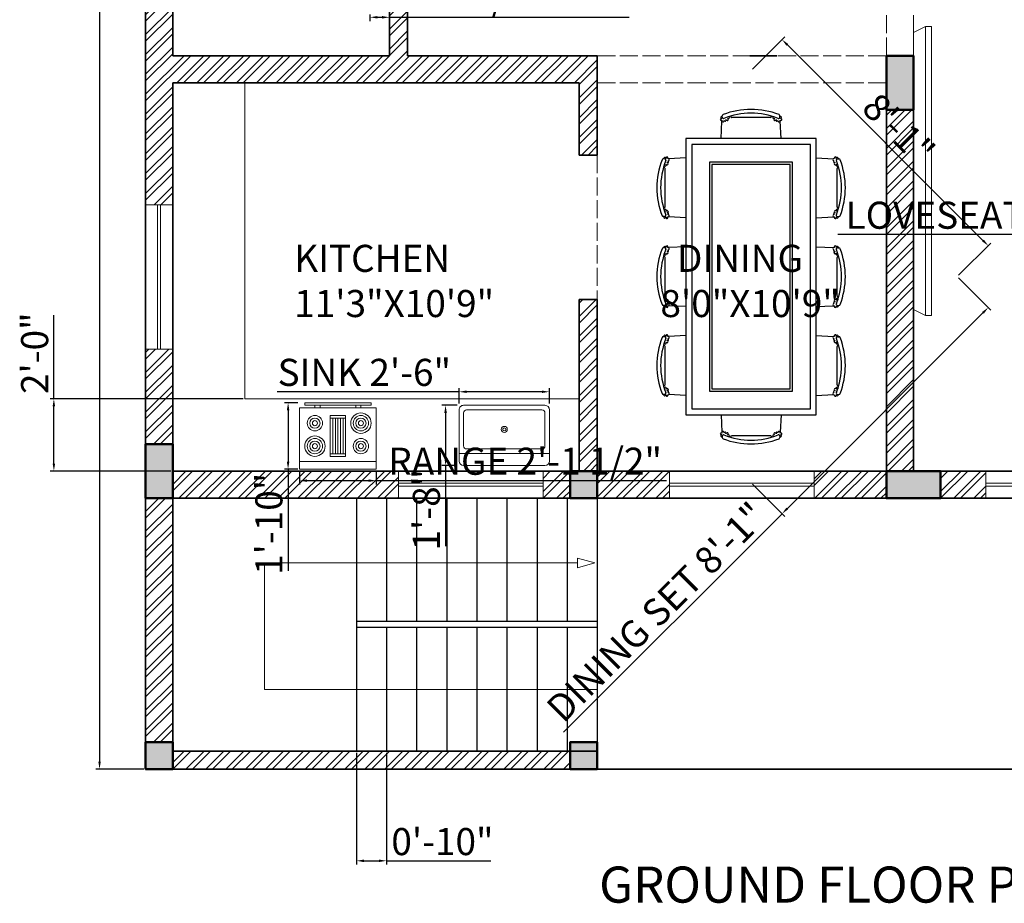
# Model space of a CAD drawing. Units: inches. Extents: x 4153 to 5577, y 785 to 1503.
# Tile 1 of 11: x 4153 to 4480, y 857 to 1150. Entities that reach past the tile are written whole.
import ezdxf

# ---------------------------------------------------------------- set-up
doc = ezdxf.new("R2010")
doc.units = ezdxf.units.IN
doc.linetypes.add('ACAD_ISO02W100', pattern=[15, 12, -3])
for name, color, linetype, lineweight in [('A-ANNO-DIMS', 2, 'Continuous', 18), ('A-ANNO-SYMB', 7, 'Continuous', 18), ('A-ANNO-TEXT', 7, 'Continuous', 35), ('A-AREA-IDEN', 7, 'Continuous', 25), ('A-COLS', 7, 'Continuous', 50), ('A-EQPM', 8, 'Continuous', 18), ('A-FLOR-CASE', 32, 'Continuous', 18), ('A-FLOR-STRS', 7, 'Continuous', 25), ('A-FURN', 8, 'Continuous', 18), ('A-GLAZ', 4, 'Continuous', 18), ('A-WALL', 7, 'Continuous', 35), ('A-WALL-OVHD', 7, 'ACAD_ISO02W100', 18), ('Сантехника', 7, 'Continuous', 18)]:
    doc.layers.add(name, color=color, linetype=linetype, lineweight=lineweight)
doc.layers.add('A-WALL-PATT', color=251, linetype='Continuous', lineweight=13, true_color=0x636466)
for name, color, linetype in [('FUR', 42, 'Continuous'), ('HA', 9, 'Continuous'), ('wood', 26, 'Continuous')]:
    doc.layers.add(name, color=color, linetype=linetype)
doc.styles.get("Standard").update_dxf_attribs({"font": 'arial.ttf'})
doc.dimstyles.new('ISO-25', dxfattribs={"dimtxt": 9, "dimasz": 2.5, "dimexe": 1.25, "dimexo": 0.625, "dimtad": 1, "dimlunit": 3, "dimtxsty": 'Standard', "dimcen": 2.5, "dimadec": 0, "dimazin": 0, "dimtfac": 1, "dimtmove": 0, "dimatfit": 3, "dimfxl": 1, "dimarcsym": 0})

# ---------------------------------------------------------------- blocks, each defined once
blk = doc.blocks.new('A$C39F63D19')
at = {"layer": 'FUR'}
for p, q in [((1.415, 2.4468), (1.4061, 2.4547)), ((1.5486, 2.3264), (1.4408, 2.4235)), ((1.3599, 2.3864), (1.1308, 2.1573)), ((1.3599, 2.4017), (1.3588, 2.4028)), ((1.8741, 2.2319), (1.9819, 2.329)), ((2.0077, 2.3522), (2.0166, 2.3602)), ((2.0628, 2.3072), (2.0639, 2.3083)), ((2.0628, 2.2919), (2.2919, 2.0628)), ((1.0705, 2.1023), (1.0625, 2.1111)), ((1.1908, 1.9686), (1.0937, 2.0765)), ((1.1155, 2.1573), (1.1144, 2.1585)), ((1.1155, 2.1573), (1.1144, 2.1585)), ((2.3072, 2.0628), (2.3083, 2.0639)), ((2.3072, 2.0628), (2.3083, 2.0639)), ((2.3522, 2.0077), (2.3602, 2.0166)), ((0.8846, 1.9165), (0.8758, 1.9244)), ((2.2319, 1.8741), (2.329, 1.9819)), ((0.8296, 1.8561), (0.6005, 1.627)), ((0.8296, 1.8714), (0.8285, 1.8725)), ((1.0183, 1.7961), (0.9104, 1.8932)), ((0.5401, 1.572), (0.5322, 1.5808)), ((0.5852, 1.627), (0.5841, 1.6281)), ((0.5852, 1.627), (0.5841, 1.6281)), ((0.6605, 1.4383), (0.5634, 1.5462)), ((2.3264, 1.5486), (2.4235, 1.4408)), ((2.4468, 1.415), (2.4547, 1.4061)), ((0.2993, 1.3411), (0.2981, 1.3422)), ((0.3543, 1.3861), (0.3455, 1.3941)), ((0.488, 1.2658), (0.3801, 1.3629)), ((2.3864, 1.3599), (2.1573, 1.1308)), ((2.4017, 1.3599), (2.4028, 1.3588)), ((0.2993, 1.3258), (0.0701, 1.0967)), ((1.9686, 1.1908), (2.0765, 1.0937)), ((0.0549, 1.0967), (0.0538, 1.0978)), ((0.0549, 1.0967), (0.0538, 1.0978)), ((2.1573, 1.1155), (2.1585, 1.1144)), ((2.1573, 1.1155), (2.1585, 1.1144)), ((0.0098, 1.0416), (0.0019, 1.0505)), ((0.1302, 0.908), (0.033, 1.0158)), ((1.7961, 1.0183), (1.8932, 0.9104)), ((2.1023, 1.0705), (2.1111, 1.0625)), ((1.9165, 0.8846), (1.9244, 0.8758)), ((1.8561, 0.8296), (1.627, 0.6005)), ((1.8714, 0.8296), (1.8725, 0.8285)), ((0.2247, 0.5825), (0.1276, 0.4747)), ((1.4383, 0.6605), (1.5462, 0.5634)), ((1.627, 0.5852), (1.6281, 0.5841)), ((1.627, 0.5852), (1.6281, 0.5841)), ((1.572, 0.5401), (1.5808, 0.5322)), ((0.1044, 0.4489), (0.0964, 0.44)), ((1.2658, 0.488), (1.3629, 0.3801)), ((0.1494, 0.3938), (0.1483, 0.3927)), ((0.1647, 0.3938), (0.3938, 0.1647)), ((1.3861, 0.3543), (1.3941, 0.3455)), ((1.3258, 0.2993), (1.0967, 0.0701)), ((1.3411, 0.2993), (1.3422, 0.2981)), ((0.5825, 0.2247), (0.4747, 0.1276)), ((0.3938, 0.1494), (0.3927, 0.1483)), ((0.3938, 0.1494), (0.3927, 0.1483)), ((0.4489, 0.1044), (0.44, 0.0964)), ((0.908, 0.1302), (1.0158, 0.033)), ((1.0416, 0.0098), (1.0505, 0.0019)), ((1.0967, 0.0549), (1.0978, 0.0538)), ((1.0967, 0.0549), (1.0978, 0.0538))]:
    blk.add_line(p, q, dxfattribs=at)
for points in [[(1.6641, 2.4419), (0.0147, 0.7925), (0.7925, 0.0147), (2.4419, 1.6641)], [(1.6641, 2.3712), (0.0854, 0.7925), (0.7925, 0.0854), (2.3712, 1.6641)], [(1.6641, 2.159), (0.2976, 0.7925), (0.7925, 0.2976), (2.159, 1.6641)]]:
    blk.add_lwpolyline(points, close=True, dxfattribs=at)
for centre, radius, start, end in [((1.6574, 1.8598), 0.6521, 113.77302, 156.22698), ((1.6574, 1.8598), 0.6197, 113.33062, 156.66938), ((1.3814, 2.4068), 0.0085, 151.04971, 5.85435), ((1.3995, 2.4044), 0.0102, 161.25601, 35.99509), ((1.3989, 2.4467), 0.0108, 48, 113.77302), ((1.4156, 2.411), 0.00785, 184.4301, 31.81325), ((1.4185, 2.4458), 0.0101, 329.62103, 147.42526), ((1.4077, 2.4388), 0.0108, 293.33062, 48), ((1.4308, 2.4208), 0.0103, 213.3009, 71.36297), ((1.4349, 2.4385), 0.00795, 264.76881, 163.65384), ((1.3523, 2.3941), 0.0108, 315, 45), ((1.9878, 2.3439), 0.00795, 16.34616, 275.23119), ((1.9919, 2.3262), 0.0103, 108.63703, 326.6991), ((2.0042, 2.3512), 0.0101, 32.57474, 210.37897), ((2.015, 2.3442), 0.0108, 132, 246.66938), ((1.7653, 1.7653), 0.6197, 23.33062, 66.66938), ((2.0238, 2.3521), 0.0108, 66.22698, 132), ((1.7653, 1.7653), 0.6521, 23.77302, 66.22698), ((2.0071, 2.3164), 0.00785, 148.18675, 355.5699), ((2.0232, 2.3098), 0.0102, 144.00491, 18.74399), ((2.0413, 2.3122), 0.0085, 174.14565, 28.95029), ((2.0704, 2.2995), 0.0108, 135, 225), ((1.0705, 2.1184), 0.0108, 156.22698, 222), ((1.0715, 2.0987), 0.0101, 122.57474, 300.37897), ((1.0785, 2.1095), 0.0108, 222, 336.66938), ((1.0788, 2.0824), 0.00795, 106.34616, 5.23119), ((1.0965, 2.0864), 0.0103, 198.63703, 56.6991), ((1.1063, 2.1017), 0.00785, 238.18675, 85.5699), ((1.1105, 2.1359), 0.0085, 264.14565, 118.95029), ((1.1232, 2.165), 0.0108, 225, 315), ((2.2995, 2.0704), 0.0108, 225, 315), ((2.3098, 2.0232), 0.0102, 71.25601, 305.99509), ((2.3122, 2.0413), 0.0085, 61.04971, 275.85435), ((2.3164, 2.0071), 0.00785, 94.4301, 301.81325), ((2.3262, 1.9919), 0.0103, 123.3009, 341.36297), ((2.3442, 2.015), 0.0108, 203.33062, 318), ((2.3439, 1.9878), 0.00795, 174.76881, 73.65384), ((2.3512, 2.0042), 0.0101, 239.62103, 57.42526), ((2.3521, 2.0238), 0.0108, 318, 23.77302), ((1.1271, 1.3295), 0.6521, 113.77302, 156.22698), ((0.8686, 1.9164), 0.0108, 48, 113.77302), ((0.8882, 1.9155), 0.0101, 329.62103, 147.42526), ((0.8774, 1.9084), 0.0108, 293.33062, 48), ((0.9045, 1.9081), 0.00795, 264.76881, 163.65384), ((1.1271, 1.3295), 0.6197, 113.33062, 156.66938), ((0.8219, 1.8638), 0.0108, 315, 45), ((0.8511, 1.8765), 0.0085, 151.04971, 5.85435), ((0.8692, 1.8741), 0.0102, 161.25601, 35.99509), ((0.8852, 1.8806), 0.00785, 184.4301, 31.81325), ((0.9005, 1.8904), 0.0103, 213.3009, 71.36297), ((0.5402, 1.588), 0.0108, 156.22698, 222), ((0.576, 1.5714), 0.00785, 238.18675, 85.5699), ((0.5801, 1.6055), 0.0085, 264.14565, 118.95029), ((0.5825, 1.5874), 0.0102, 234.00491, 108.74399), ((0.5928, 1.6347), 0.0108, 225, 315), ((0.5411, 1.5684), 0.0101, 122.57474, 300.37897), ((0.5482, 1.5792), 0.0108, 222, 336.66938), ((0.5485, 1.5521), 0.00795, 106.34616, 5.23119), ((0.5662, 1.5561), 0.0103, 198.63703, 56.6991), ((1.8598, 1.6574), 0.6197, 293.33062, 336.66938), ((2.411, 1.4156), 0.00785, 58.18675, 265.5699), ((2.4208, 1.4308), 0.0103, 18.63703, 236.6991), ((2.4388, 1.4077), 0.0108, 42, 156.66938), ((2.4385, 1.4349), 0.00795, 286.34616, 185.23119), ((2.4458, 1.4185), 0.0101, 302.57474, 120.37897), ((0.5968, 0.7992), 0.6521, 113.77302, 156.22698), ((0.5968, 0.7992), 0.6197, 113.33062, 156.66938), ((0.2916, 1.3334), 0.0108, 315, 45), ((0.3207, 1.3461), 0.0085, 151.04971, 5.85435), ((0.3388, 1.3437), 0.0102, 161.25601, 35.99509), ((0.3382, 1.3861), 0.0108, 48, 113.77302), ((0.3549, 1.3503), 0.00785, 184.4301, 31.81325), ((0.3579, 1.3851), 0.0101, 329.62103, 147.42526), ((0.3471, 1.3781), 0.0108, 293.33062, 48), ((0.3702, 1.3601), 0.0103, 213.3009, 71.36297), ((0.3742, 1.3778), 0.00795, 264.76881, 163.65384), ((1.8598, 1.6574), 0.6521, 293.77302, 336.22698), ((2.3941, 1.3523), 0.0108, 45, 135), ((2.4044, 1.3995), 0.0102, 54.00491, 288.74399), ((2.4068, 1.3814), 0.0085, 84.14565, 298.95029), ((2.4467, 1.3989), 0.0108, 336.22698, 42), ((0.0498, 1.0752), 0.0085, 264.14565, 118.95029), ((0.0625, 1.1043), 0.0108, 225, 315), ((2.0824, 1.0788), 0.00795, 84.76881, 343.65384), ((2.0864, 1.0965), 0.0103, 33.3009, 251.36297), ((2.1017, 1.1063), 0.00785, 4.4301, 211.81325), ((2.1095, 1.0785), 0.0108, 113.33062, 228), ((2.1178, 1.1129), 0.0102, 341.25601, 215.99509), ((2.1359, 1.1105), 0.0085, 331.04971, 185.85435), ((2.165, 1.1232), 0.0108, 135, 225), ((0.0099, 1.0577), 0.0108, 156.22698, 222), ((0.0108, 1.0381), 0.0101, 122.57474, 300.37897), ((0.0178, 1.0489), 0.0108, 222, 336.66938), ((0.0181, 1.0217), 0.00795, 106.34616, 5.23119), ((0.0358, 1.0258), 0.0103, 198.63703, 56.6991), ((0.0456, 1.041), 0.00785, 238.18675, 85.5699), ((0.0522, 1.0571), 0.0102, 234.00491, 108.74399), ((2.0987, 1.0715), 0.0101, 149.62103, 327.42526), ((2.1184, 1.0705), 0.0108, 228, 293.77302), ((1.3295, 1.1271), 0.6197, 293.33062, 336.66938), ((1.3295, 1.1271), 0.6521, 293.77302, 336.22698), ((1.8638, 0.8219), 0.0108, 45, 135), ((1.8741, 0.8692), 0.0102, 54.00491, 288.74399), ((1.8765, 0.8511), 0.0085, 84.14565, 298.95029), ((1.8806, 0.8852), 0.00785, 58.18675, 265.5699), ((1.8904, 0.9005), 0.0103, 18.63703, 236.6991), ((1.9084, 0.8774), 0.0108, 42, 156.66938), ((1.9081, 0.9045), 0.00795, 286.34616, 185.23119), ((1.9155, 0.8882), 0.0101, 302.57474, 120.37897), ((1.9164, 0.8686), 0.0108, 336.22698, 42), ((1.5714, 0.576), 0.00785, 4.4301, 211.81325), ((1.5874, 0.5825), 0.0102, 341.25601, 215.99509), ((1.6055, 0.5801), 0.0085, 331.04971, 185.85435), ((1.6347, 0.5928), 0.0108, 135, 225), ((1.5521, 0.5485), 0.00795, 84.76881, 343.65384), ((1.5561, 0.5662), 0.0103, 33.3009, 251.36297), ((1.5684, 0.5411), 0.0101, 149.62103, 327.42526), ((1.5792, 0.5482), 0.0108, 113.33062, 228), ((1.588, 0.5402), 0.0108, 228, 293.77302), ((0.1044, 0.4328), 0.0108, 138, 203.77302), ((0.6913, 0.6913), 0.6521, 203.77302, 246.22698), ((0.1054, 0.4524), 0.0101, 59.62103, 237.42526), ((0.1124, 0.4416), 0.0108, 23.33062, 138), ((0.1127, 0.4688), 0.00795, 354.76881, 253.65384), ((0.1304, 0.4647), 0.0103, 303.3009, 161.36297), ((0.6913, 0.6913), 0.6197, 203.33062, 246.66938), ((0.1402, 0.4495), 0.00785, 274.4301, 121.81325), ((0.1444, 0.4153), 0.0085, 241.04971, 95.85435), ((0.1468, 0.4334), 0.0102, 251.25601, 125.99509), ((0.1571, 0.3862), 0.0108, 45, 135), ((0.7992, 0.5968), 0.6197, 293.33062, 336.66938), ((0.7992, 0.5968), 0.6521, 293.77302, 336.22698), ((1.3437, 0.3388), 0.0102, 54.00491, 288.74399), ((1.3503, 0.3549), 0.00785, 58.18675, 265.5699), ((1.3601, 0.3702), 0.0103, 18.63703, 236.6991), ((1.3781, 0.3471), 0.0108, 42, 156.66938), ((1.3778, 0.3742), 0.00795, 286.34616, 185.23119), ((1.3851, 0.3579), 0.0101, 302.57474, 120.37897), ((1.3861, 0.3382), 0.0108, 336.22698, 42), ((1.3334, 0.2916), 0.0108, 45, 135), ((1.3461, 0.3207), 0.0085, 84.14565, 298.95029), ((0.3862, 0.1571), 0.0108, 315, 45), ((0.4153, 0.1444), 0.0085, 354.14565, 208.95029), ((0.4334, 0.1468), 0.0102, 324.00491, 198.74399), ((0.4328, 0.1044), 0.0108, 246.22698, 312), ((0.4495, 0.1402), 0.00785, 328.18675, 175.5699), ((0.4524, 0.1054), 0.0101, 212.57474, 30.37897), ((0.4416, 0.1124), 0.0108, 312, 66.66938), ((0.4647, 0.1304), 0.0103, 288.63703, 146.6991), ((0.4688, 0.1127), 0.00795, 196.34616, 95.23119), ((1.0217, 0.0181), 0.00795, 84.76881, 343.65384), ((1.0258, 0.0358), 0.0103, 33.3009, 251.36297), ((1.0381, 0.0108), 0.0101, 149.62103, 327.42526), ((1.041, 0.0456), 0.00785, 4.4301, 211.81325), ((1.0489, 0.0178), 0.0108, 113.33062, 228), ((1.0571, 0.0522), 0.0102, 341.25601, 215.99509), ((1.0577, 0.0099), 0.0108, 228, 293.77302), ((1.0752, 0.0498), 0.0085, 331.04971, 185.85435), ((1.1043, 0.0625), 0.0108, 135, 225)]:
    blk.add_arc(centre, radius, start, end, dxfattribs=at)
at = {"layer": 'HA'}
blk.add_lwpolyline([(1.6641, 2.1308), (0.3258, 0.7925), (0.7925, 0.3258), (2.1308, 1.6641)], close=True, dxfattribs=at)
at = {"layer": 'wood'}
for points in [[(1.3825, 2.4152, 0.308332), (1.374, 2.4109, -0.00386)], [(1.4096, 2.4059, -0.15729), (1.4077, 2.4104, -0.120016)], [(1.1113, 2.1077, 1.044756), (1.1135, 2.1279, -0.117685), (1.1096, 2.1274, -1.643727), (1.1069, 2.1095, -0.15729)], [(2.3158, 2.015, -0.120016), (2.3113, 2.0131, -0.15729)], [(0.8522, 1.8849, 0.308332), (0.8436, 1.8806, -0.00386)], [(0.8792, 1.8756, -0.15729), (0.8774, 1.88, -0.120016)], [(0.581, 1.5774, 1.044756), (0.5832, 1.5976, -0.117685), (0.5793, 1.5971, -1.643727), (0.5766, 1.5792, -0.15729)], [(0.3489, 1.3453, -0.15729), (0.3471, 1.3497, -0.120016)], [(2.4104, 1.4077, -0.15729), (2.4059, 1.4096, 1.044756), (2.4037, 1.3893, -0.117685), (2.4077, 1.3899, -1.643727)], [(2.1095, 1.1069, -0.120016), (2.1077, 1.1113, -0.15729)], [(2.1347, 1.102, 0.308332), (2.1433, 1.1064, -0.00386)], [(1.88, 0.8774, -0.15729), (1.8756, 0.8792, 1.044756), (1.8734, 0.859, -0.117685), (1.8773, 0.8595, -1.643727)], [(1.5792, 0.5766, -0.120016), (1.5774, 0.581, -0.15729)], [(1.6044, 0.5717, 0.308332), (1.613, 0.576, -0.00386)], [(0.1453, 0.4435, -0.15729), (0.1408, 0.4416, -0.120016)], [(1.3497, 0.3471, -0.15729), (1.3453, 0.3489, 1.044756), (1.3431, 0.3287, -0.117685), (1.347, 0.3292, -1.643727)], [(1.0489, 0.0462, -0.120016), (1.047, 0.0507, -0.15729)], [(1.0741, 0.0414, 0.308332), (1.0826, 0.0457, -0.00386)]]:
    blk.add_lwpolyline(points, format="xyb", close=True, dxfattribs=at)
blk = doc.blocks.new('Range-Oven - 30 in top')
for p, q in [((0, -3), (30, -3)), ((12, -6), (18, -6)), ((13, -20), (13, -6)), ((14, -6), (14, -20)), ((15, -20), (15, -6)), ((16, -6), (16, -20)), ((17, -20), (17, -6)), ((18, -20), (12, -20)), ((6, -24), (6, -25)), ((8, -25), (8, -24)), ((22, -25), (22, -24)), ((24, -24), (24, -25))]:
    blk.add_line(p, q)
for points in [[(0, -24), (0, 0), (30, 0), (30, -24)], [(12, -21), (12, -5), (18, -5), (18, -21)], [(2, -26), (2, -25), (28, -25), (28, -26)]]:
    blk.add_lwpolyline(points, close=True)
for centre, radius in [((6, -9), 4), ((6, -9), 3), ((6, -9), 2), ((24, -9), 3), ((24, -9), 2), ((6, -9), 1), ((24, -9), 1), ((6, -18), 3), ((24, -18), 4), ((24, -18), 3), ((6, -18), 2), ((6, -18), 1), ((24, -18), 2), ((24, -18), 1)]:
    blk.add_circle(centre, radius)
blk = doc.blocks.new('Sink-single - 30 in top')
blk.add_line((-15, -3.999996), (15, -3.999996))
for points in [[(-13.5, 0), (13.5, 0)], [(-15, -18.499996), (-15, -1.5)], [(15, -1.5), (15, -18.499996)], [(-13.5, -17.499996), (-13.5, -6.499996)], [(-12.5, -5.499996), (12.5, -5.499996)], [(13.5, -6.499996), (13.5, -17.499996)], [(12.5, -18.499996), (-12.5, -18.499996)], [(13.5, -19.999996), (-13.5, -19.999996)]]:
    blk.add_lwpolyline(points)
for radius in [1, 0.5]:
    blk.add_circle((0, -11.999996), radius)
for centre, radius, start, end in [((-13.5, -1.5), 1.5, 90, 180), ((13.5, -1.5), 1.5, 0, 90), ((-12.5, -6.499996), 1, 90, 180), ((12.5, -6.499996), 1, 0, 90), ((-13.5, -18.499996), 1.5, 180, 270), ((-12.5, -17.499996), 1, 180, 270), ((12.5, -17.499996), 1, 270, 0), ((13.5, -18.499996), 1.5, 270, 0)]:
    blk.add_arc(centre, radius, start, end)
blk = doc.blocks.new('*D22')
at = {"layer": 'A-ANNO-DIMS', "color": 0, "lineweight": -2, "transparency": 16777216}
for p, q in [((4194.3, 1444.49), (4178.39, 1444.49)), ((4179.64, 1441.99), (4179.64, 903.99)), ((4194.3, 901.49), (4178.39, 901.49))]:
    blk.add_line(p, q, dxfattribs=at)
at = {"layer": 'A-ANNO-DIMS', "color": 0, "transparency": 16777216}
for points in [[(4179.23, 1441.99), (4180.06, 1441.99), (4179.64, 1444.49)], [(4179.23, 903.99), (4180.06, 903.99), (4179.64, 901.49)]]:
    blk.add_solid(points, dxfattribs=at)
at = {"layer": 'Defpoints', "color": 0, "transparency": 16777216}
for p in [(4194.93, 1444.49), (4179.64, 901.49), (4194.93, 901.49)]:
    blk.add_point(p, dxfattribs=at)
at = {"layer": 'A-ANNO-DIMS', "color": 0, "transparency": 16777216, "insert": (4174.42, 1172.99), "char_height": 9, "attachment_point": 5, "rotation": 90}
blk.add_mtext('45\'-3"', dxfattribs=at)
blk = doc.blocks.new('WINDOW-48IN')
for p, q in [((0, 9), (0, 0)), ((48, 9), (48, 0)), ((0, 5), (48, 5)), ((0, 4), (48, 4))]:
    blk.add_line(p, q)
blk = doc.blocks.new('WINDOW-72IN')
for p, q in [((0, 9), (0, 0)), ((72, 9), (72, 0)), ((0, 5), (72, 5)), ((0, 4), (72, 4))]:
    blk.add_line(p, q)
blk = doc.blocks.new('COL-9X18IN')
at = {"transparency": 33554687}
h = blk.add_hatch(color=256, dxfattribs=at)
h.dxf.hatch_style = 1
h.paths.add_polyline_path([(9, 18), (0, 18), (0, 0), (9, 0)])
blk.add_lwpolyline([(0, 18), (9, 18), (9, 0), (0, 0)], close=True)
blk = doc.blocks.new('COL-9X9IN')
at = {"transparency": 33554687}
h = blk.add_hatch(color=256, dxfattribs=at)
h.dxf.hatch_style = 1
h.paths.add_polyline_path([(9, 0), (9, 9), (0, 9), (0, 0)])
blk.add_lwpolyline([(0, 9), (9, 9), (9, 0), (0, 0)], close=True)
blk = doc.blocks.new('SITOUT-RETURN-STAIR')
at = {"ltscale": 0.5}
for p, q in [((0, 84), (0, 41)), ((10, 84), (10, 43)), ((20, 84), (20, 43)), ((30, 84), (30, 43)), ((40, 84), (40, 43)), ((50, 84), (50, 43)), ((60, 84), (60, 43)), ((70, 84), (70, 43)), ((80, 84), (80, 41))]:
    blk.add_line(p, q, dxfattribs=at)
for p, q in [((80, 43), (0, 43)), ((80, 41), (0, 41)), ((0, 41), (0, 0)), ((10, 41), (10, 0)), ((20, 41), (20, 0)), ((30, 41), (30, 0)), ((40, 41), (40, 0)), ((50, 41), (50, 0)), ((60, 41), (60, 0)), ((70, 41), (70, 0)), ((80, 41), (80, 0))]:
    blk.add_line(p, q)
blk = doc.blocks.new('STAIR-DIRECTION-RETURN')
at = {"ltscale": 0.5}
for p, q in [((103.89, 42), (0, 42)), ((0, 0), (0, 42)), ((110.5, 0), (0, 0))]:
    blk.add_line(p, q, dxfattribs=at)
blk.add_lwpolyline([(109.65, 42), (103.89, 43.63), (103.89, 40.37)], close=True)
blk = doc.blocks.new('*D117')
at = {"layer": 'A-ANNO-DIMS', "color": 0, "lineweight": -2, "transparency": 16777216}
for p, q in [((4269.43, 1152.11), (4269.43, 1149.99)), ((4271.93, 1151.24), (4273.43, 1151.24)), ((4275.93, 1152.11), (4275.93, 1149.99)), ((4275.93, 1151.24), (4355.51, 1151.24))]:
    blk.add_line(p, q, dxfattribs=at)
at = {"layer": 'A-ANNO-DIMS', "color": 0, "transparency": 16777216}
for points in [[(4271.93, 1151.66), (4271.93, 1150.82), (4269.43, 1151.24)], [(4273.43, 1151.66), (4273.43, 1150.82), (4275.93, 1151.24)]]:
    blk.add_solid(points, dxfattribs=at)
at = {"layer": 'Defpoints', "color": 0, "transparency": 16777216}
for p in [(4269.43, 1152.74), (4275.93, 1152.74), (4275.93, 1151.24)]:
    blk.add_point(p, dxfattribs=at)
at = {"layer": 'A-ANNO-DIMS', "color": 0, "transparency": 16777216, "insert": (4316.97, 1156.52), "char_height": 9, "attachment_point": 5}
blk.add_mtext('0\'-6 1/2" TYP.', dxfattribs=at)
blk = doc.blocks.new('*D124')
at = {"layer": 'A-ANNO-DIMS', "color": 0, "lineweight": -2, "transparency": 16777216}
for p, q in [((4542.96, 1079.04), (4424.83, 1079.04)), ((4542.96, 1070.29), (4542.96, 1080.29)), ((4602.94, 1079.04), (4545.46, 1079.04)), ((4605.44, 1070.29), (4605.44, 1080.29))]:
    blk.add_line(p, q, dxfattribs=at)
at = {"layer": 'A-ANNO-DIMS', "color": 0, "transparency": 16777216}
for points in [[(4545.46, 1079.46), (4545.46, 1078.63), (4542.96, 1079.04)], [(4602.94, 1079.46), (4602.94, 1078.63), (4605.44, 1079.04)]]:
    blk.add_solid(points, dxfattribs=at)
at = {"layer": 'Defpoints', "color": 0, "transparency": 16777216}
for p in [(4542.96, 1079.04), (4542.96, 1069.67), (4605.44, 1069.67)]:
    blk.add_point(p, dxfattribs=at)
at = {"layer": 'A-ANNO-DIMS', "color": 0, "transparency": 16777216, "insert": (4482.65, 1084.32), "char_height": 9, "attachment_point": 5}
blk.add_mtext('LOVESEAT 5\'-2 1/2"', dxfattribs=at)
blk = doc.blocks.new('*D134')
at = {"layer": 'A-ANNO-DIMS', "color": 0, "lineweight": -2, "transparency": 16777216}
for p, q in [((4464.93, 1064.64), (4475.65, 1053.93)), ((4472.99, 1053.04), (4408.05, 988.09)), ((4396.45, 996.16), (4407.16, 985.44)), ((4406.28, 986.33), (4333.68, 913.73))]:
    blk.add_line(p, q, dxfattribs=at)
at = {"layer": 'A-ANNO-DIMS', "color": 0, "transparency": 16777216}
for points in [[(4472.7, 1053.34), (4473.29, 1052.75), (4474.76, 1054.81)], [(4407.75, 988.39), (4408.34, 987.8), (4406.28, 986.33)]]:
    blk.add_solid(points, dxfattribs=at)
at = {"layer": 'Defpoints', "color": 0, "transparency": 16777216}
for p in [(4464.49, 1065.08), (4396.01, 996.6), (4406.28, 986.33)]:
    blk.add_point(p, dxfattribs=at)
at = {"layer": 'A-ANNO-DIMS', "color": 0, "transparency": 16777216, "insert": (4365.36, 952.88), "char_height": 9, "attachment_point": 5, "rotation": 45}
blk.add_mtext('DINING SET 8\'-1"', dxfattribs=at)
blk = doc.blocks.new('*D135')
at = {"layer": 'A-ANNO-DIMS', "color": 0, "lineweight": -2, "transparency": 16777216}
for p, q in [((4396.45, 1134.01), (4407.16, 1144.72)), ((4408.05, 1142.07), (4472.99, 1077.12)), ((4464.93, 1065.53), (4475.65, 1076.24))]:
    blk.add_line(p, q, dxfattribs=at)
at = {"layer": 'A-ANNO-DIMS', "color": 0, "transparency": 16777216}
for points in [[(4408.34, 1142.37), (4407.75, 1141.78), (4406.28, 1143.84)], [(4473.29, 1077.42), (4472.7, 1076.83), (4474.76, 1075.36)]]:
    blk.add_solid(points, dxfattribs=at)
at = {"layer": 'Defpoints', "color": 0, "transparency": 16777216}
for p in [(4396.01, 1133.57), (4474.76, 1075.36), (4464.49, 1065.08)]:
    blk.add_point(p, dxfattribs=at)
at = {"layer": 'A-ANNO-DIMS', "color": 0, "transparency": 16777216, "insert": (4444.21, 1113.29), "char_height": 9, "attachment_point": 5, "rotation": 315}
blk.add_mtext('8\'-1"', dxfattribs=at)
blk = doc.blocks.new('*D136')
at = {"layer": 'A-ANNO-DIMS', "color": 0, "lineweight": -2, "transparency": 16777216}
for p, q in [((4246.08, 1000.52), (4246.08, 996.07)), ((4248.58, 997.32), (4269.03, 997.32)), ((4271.53, 1000.52), (4271.53, 996.07)), ((4271.53, 997.32), (4367.92, 997.32))]:
    blk.add_line(p, q, dxfattribs=at)
at = {"layer": 'A-ANNO-DIMS', "color": 0, "transparency": 16777216}
for points in [[(4248.58, 997.74), (4248.58, 996.91), (4246.08, 997.32)], [(4269.03, 997.74), (4269.03, 996.91), (4271.53, 997.32)]]:
    blk.add_solid(points, dxfattribs=at)
at = {"layer": 'Defpoints', "color": 0, "transparency": 16777216}
for p in [(4246.08, 1001.14), (4271.53, 1001.14), (4271.53, 997.32)]:
    blk.add_point(p, dxfattribs=at)
at = {"layer": 'A-ANNO-DIMS', "color": 0, "transparency": 16777216, "insert": (4320.97, 1002.6), "char_height": 9, "attachment_point": 5}
blk.add_mtext('RANGE 2\'-1 1/2"', dxfattribs=at)
blk = doc.blocks.new('*D137')
at = {"layer": 'A-ANNO-DIMS', "color": 0, "lineweight": -2, "transparency": 16777216}
for p, q in [((4245.45, 1023.2), (4241.01, 1023.2)), ((4242.26, 1020.7), (4242.26, 1003.64)), ((4245.45, 1001.14), (4241.01, 1001.14)), ((4242.26, 1001.14), (4242.26, 967.32))]:
    blk.add_line(p, q, dxfattribs=at)
at = {"layer": 'A-ANNO-DIMS', "color": 0, "transparency": 16777216}
for points in [[(4241.84, 1020.7), (4242.67, 1020.7), (4242.26, 1023.2)], [(4241.84, 1003.64), (4242.67, 1003.64), (4242.26, 1001.14)]]:
    blk.add_solid(points, dxfattribs=at)
at = {"layer": 'Defpoints', "color": 0, "transparency": 16777216}
for p in [(4246.08, 1023.2), (4242.26, 1001.14), (4246.08, 1001.14)]:
    blk.add_point(p, dxfattribs=at)
at = {"layer": 'A-ANNO-DIMS', "color": 0, "transparency": 16777216, "insert": (4237.04, 982.98), "char_height": 9, "attachment_point": 5, "rotation": 90}
blk.add_mtext('1\'-10"', dxfattribs=at)
blk = doc.blocks.new('*D138')
at = {"layer": 'A-ANNO-DIMS', "color": 0, "lineweight": -2, "transparency": 16777216}
for p, q in [((4299.05, 1026.84), (4238.58, 1026.84)), ((4299.05, 1022.97), (4299.05, 1028.09)), ((4326.55, 1026.84), (4301.55, 1026.84)), ((4329.05, 1022.97), (4329.05, 1028.09))]:
    blk.add_line(p, q, dxfattribs=at)
at = {"layer": 'A-ANNO-DIMS', "color": 0, "transparency": 16777216}
for points in [[(4301.55, 1027.26), (4301.55, 1026.43), (4299.05, 1026.84)], [(4326.55, 1027.26), (4326.55, 1026.43), (4329.05, 1026.84)]]:
    blk.add_solid(points, dxfattribs=at)
at = {"layer": 'Defpoints', "color": 0, "transparency": 16777216}
for p in [(4299.05, 1026.84), (4299.05, 1022.34), (4329.05, 1022.34)]:
    blk.add_point(p, dxfattribs=at)
at = {"layer": 'A-ANNO-DIMS', "color": 0, "transparency": 16777216, "insert": (4267.57, 1032.12), "char_height": 9, "attachment_point": 5}
blk.add_mtext('SINK 2\'-6"', dxfattribs=at)
blk = doc.blocks.new('*D139')
at = {"layer": 'A-ANNO-DIMS', "color": 0, "lineweight": -2, "transparency": 16777216}
for p, q in [((4298.43, 1022.34), (4293.3, 1022.34)), ((4294.55, 1019.84), (4294.55, 1004.84)), ((4298.43, 1002.34), (4293.3, 1002.34)), ((4294.55, 1002.34), (4294.55, 975.52))]:
    blk.add_line(p, q, dxfattribs=at)
at = {"layer": 'A-ANNO-DIMS', "color": 0, "transparency": 16777216}
for points in [[(4294.13, 1019.84), (4294.97, 1019.84), (4294.55, 1022.34)], [(4294.13, 1004.84), (4294.97, 1004.84), (4294.55, 1002.34)]]:
    blk.add_solid(points, dxfattribs=at)
at = {"layer": 'Defpoints', "color": 0, "transparency": 16777216}
for p in [(4299.05, 1022.34), (4294.55, 1002.34), (4299.05, 1002.34)]:
    blk.add_point(p, dxfattribs=at)
at = {"layer": 'A-ANNO-DIMS', "color": 0, "transparency": 16777216, "insert": (4289.33, 987.68), "char_height": 9, "attachment_point": 5, "rotation": 90}
blk.add_mtext('1\'-8"', dxfattribs=at)
blk = doc.blocks.new('*D159')
at = {"layer": 'A-ANNO-DIMS', "color": 0, "lineweight": -2, "transparency": 16777216}
for p, q in [((4264.93, 906.86), (4264.93, 869.79)), ((4274.93, 906.86), (4274.93, 869.79)), ((4267.43, 871.04), (4272.43, 871.04)), ((4274.93, 871.04), (4309.59, 871.04))]:
    blk.add_line(p, q, dxfattribs=at)
at = {"layer": 'A-ANNO-DIMS', "color": 0, "transparency": 16777216}
for points in [[(4267.43, 871.46), (4267.43, 870.62), (4264.93, 871.04)], [(4272.43, 871.46), (4272.43, 870.62), (4274.93, 871.04)]]:
    blk.add_solid(points, dxfattribs=at)
at = {"layer": 'Defpoints', "color": 0, "transparency": 16777216}
for p in [(4264.93, 907.49), (4274.93, 907.49), (4274.93, 871.04)]:
    blk.add_point(p, dxfattribs=at)
at = {"layer": 'A-ANNO-DIMS', "color": 0, "transparency": 16777216, "insert": (4293.51, 876.26), "char_height": 9, "attachment_point": 5}
blk.add_mtext('0\'-10"', dxfattribs=at)
blk = doc.blocks.new('*D160')
at = {"layer": 'A-ANNO-DIMS', "color": 0, "lineweight": -2, "transparency": 16777216}
for p, q in [((4164.48, 1024.49), (4164.48, 1052.32)), ((4227.3, 1024.49), (4163.23, 1024.49)), ((4164.48, 1002.99), (4164.48, 1021.99)), ((4203.3, 1000.49), (4163.23, 1000.49))]:
    blk.add_line(p, q, dxfattribs=at)
at = {"layer": 'A-ANNO-DIMS', "color": 0, "transparency": 16777216}
for points in [[(4164.06, 1021.99), (4164.89, 1021.99), (4164.48, 1024.49)], [(4164.06, 1002.99), (4164.89, 1002.99), (4164.48, 1000.49)]]:
    blk.add_solid(points, dxfattribs=at)
at = {"layer": 'Defpoints', "color": 0, "transparency": 16777216}
for p in [(4164.48, 1024.49), (4227.93, 1024.49), (4203.93, 1000.49)]:
    blk.add_point(p, dxfattribs=at)
at = {"layer": 'A-ANNO-DIMS', "color": 0, "transparency": 16777216, "insert": (4159.26, 1039.65), "char_height": 9, "attachment_point": 5, "rotation": 90}
blk.add_mtext('2\'-0"', dxfattribs=at)

msp = doc.modelspace()

# ---------------------------------------------------------------- hatches: boundary and pattern name
at = {"layer": 'A-WALL-PATT', "transparency": 33554687}
h = msp.add_hatch(dxfattribs=at)
h.set_pattern_fill('ANSI32', color=256, scale=0.49)
h.paths.add_polyline_path([(4344.927, 1138.488), (4281.927, 1138.488), (4281.927, 1234.488), (4296.927, 1234.488), (4296.927, 1243.488), (4269.927, 1243.488), (4269.927, 1234.488), (4275.927, 1234.488), (4275.927, 1138.488), (4203.927, 1138.488), (4203.927, 1168.488), (4194.927, 1168.488), (4194.927, 1088.988), (4203.927, 1088.988), (4203.927, 1129.488), (4338.927, 1129.488), (4338.927, 1105.488), (4344.927, 1105.488)])
h.paths.add_polyline_path([(4203.927, 1040.988), (4194.927, 1040.988), (4194.927, 1009.488), (4203.927, 1009.488)])
h.paths.add_polyline_path([(4278.927, 1000.488), (4203.927, 1000.488), (4203.927, 991.488), (4278.927, 991.488)])
h.paths.add_polyline_path([(4203.927, 991.488), (4194.927, 991.488), (4194.927, 910.488), (4203.927, 910.488)])
h.paths.add_polyline_path([(4335.927, 907.488), (4203.927, 907.488), (4203.927, 901.488), (4335.927, 901.488)])
h.paths.add_polyline_path([(4344.927, 1057.488), (4338.927, 1057.488), (4338.927, 1000.488), (4344.927, 1000.488)])
h.paths.add_polyline_path([(4335.927, 1000.488), (4326.927, 1000.488), (4326.927, 991.488), (4335.927, 991.488)])
h.paths.add_polyline_path([(4368.927, 1000.488), (4344.927, 1000.488), (4344.927, 991.488), (4368.927, 991.488)])
h.paths.add_polyline_path([(4440.927, 1000.488), (4416.927, 1000.488), (4416.927, 991.488), (4440.927, 991.488)])
h.paths.add_polyline_path([(4449.927, 1120.488), (4440.927, 1120.488), (4440.927, 1000.488), (4449.927, 1000.488)])
h.paths.add_polyline_path([(4473.927, 1000.488), (4458.927, 1000.488), (4458.927, 991.488), (4473.927, 991.488)])
h.paths.add_polyline_path([(4638.927, 1000.488), (4545.927, 1000.488), (4545.927, 991.488), (4638.927, 991.488)])
h.paths.add_polyline_path([(4701.927, 1036.488), (4692.927, 1036.488), (4692.927, 1009.488), (4701.927, 1009.488)])
h.paths.add_polyline_path([(4692.927, 1000.488), (4686.927, 1000.488), (4686.927, 991.488), (4692.927, 991.488)])
h.paths.add_polyline_path([(4701.927, 1132.488), (4692.927, 1132.488), (4692.927, 1108.488), (4701.927, 1108.488)])
h.paths.add_polyline_path([(4701.927, 1225.488), (4692.927, 1225.488), (4692.927, 1204.488), (4701.927, 1204.488)])
h.paths.add_polyline_path([(4650.927, 1243.488), (4560.927, 1243.488), (4560.927, 1265.228), (4560.927, 1381.488), (4650.927, 1381.488), (4650.927, 1393.488), (4644.927, 1393.488), (4644.927, 1387.488), (4560.927, 1387.488), (4560.927, 1435.488), (4551.927, 1435.488), (4551.927, 1354.488), (4530.927, 1354.488), (4530.927, 1348.488), (4551.927, 1348.488), (4551.927, 1309.488), (4485.927, 1309.488), (4485.927, 1234.488), (4505.427, 1234.488), (4505.427, 1243.488), (4494.927, 1243.488), (4494.927, 1303.488), (4551.927, 1303.488), (4551.927, 1243.488), (4541.427, 1243.488), (4541.427, 1234.488), (4650.927, 1234.488)])
h.paths.add_polyline_path([(4701.927, 1426.488), (4692.927, 1426.488), (4692.927, 1357.488), (4701.927, 1357.488)])
h.paths.add_polyline_path([(4701.927, 1309.488), (4692.927, 1309.488), (4692.927, 1243.488), (4701.927, 1243.488)])
h.paths.add_polyline_path([(4692.927, 1444.488), (4608.927, 1444.488), (4608.927, 1435.488), (4644.927, 1435.488), (4644.927, 1423.488), (4650.927, 1423.488), (4650.927, 1435.488), (4692.927, 1435.488)])
h.paths.add_polyline_path([(4497.927, 1444.488), (4479.927, 1444.488), (4479.927, 1435.488), (4485.927, 1435.488), (4485.927, 1348.488), (4500.927, 1348.488), (4500.927, 1354.488), (4494.927, 1354.488), (4494.927, 1435.488), (4497.927, 1435.488)])
h.paths.add_polyline_path([(4551.927, 1444.488), (4545.927, 1444.488), (4545.927, 1435.488), (4551.927, 1435.488)])
h.paths.add_polyline_path([(4572.927, 1444.488), (4569.927, 1444.488), (4569.927, 1435.488), (4572.927, 1435.488)])
h.paths.add_polyline_path([(4431.927, 1444.488), (4356.927, 1444.488), (4356.927, 1435.488), (4431.927, 1435.488)])
h.paths.add_polyline_path([(4284.927, 1444.488), (4203.927, 1444.488), (4203.927, 1435.488), (4284.927, 1435.488)])
h.paths.add_polyline_path([(4203.927, 1426.488), (4194.927, 1426.488), (4194.927, 1293.488), (4203.927, 1293.488), (4203.927, 1295.242)])
h.paths.add_polyline_path([(4347.927, 1435.488), (4338.927, 1435.488), (4338.927, 1243.488), (4332.927, 1243.488), (4332.927, 1234.488), (4431.927, 1234.488), (4431.927, 1243.488), (4347.927, 1243.488)])
h.paths.add_polyline_path([(4239.927, 1243.488), (4203.927, 1243.488), (4203.927, 1234.488), (4239.927, 1234.488)], flags=17)
h.paths.add_polyline_path([(4203.927, 1225.488), (4194.927, 1225.488), (4194.927, 1198.488), (4203.927, 1198.488)], flags=17)

# ---------------------------------------------------------------- linework, layer by layer
at = {"layer": 'A-EQPM'}
for p, q in [((4453.927, 1148.145), (4449.927, 1146.145)), ((4453.927, 1148.145), (4455.927, 1148.145)), ((4453.927, 1148.145), (4453.927, 1052.145)), ((4455.927, 1148.145), (4455.927, 1052.145)), ((4449.927, 1054.145), (4449.927, 1146.145)), ((4449.927, 1054.145), (4453.927, 1052.145)), ((4455.927, 1052.145), (4453.927, 1052.145))]:
    msp.add_line(p, q, dxfattribs=at)
at = {"layer": 'A-FLOR-CASE'}
for q in [(4227.927, 1129.488), (4338.927, 1024.488)]:
    msp.add_line((4227.927, 1024.488), q, dxfattribs=at)
at = {"layer": 'A-WALL'}
for p, q in [((4194.927, 901.488), (4194.927, 1444.488)), ((4203.927, 1138.488), (4203.927, 1234.488)), ((4275.927, 1138.488), (4275.927, 1234.488)), ((4281.927, 1138.488), (4281.927, 1234.488)), ((4203.927, 1138.488), (4275.927, 1138.488)), ((4281.927, 1138.488), (4344.927, 1138.488)), ((4344.927, 1105.488), (4344.927, 1138.488)), ((4395.573, 1138.488), (4404.573, 1138.488)), ((4440.927, 1000.488), (4440.927, 1138.488)), ((4440.927, 1138.488), (4449.927, 1138.488)), ((4449.927, 1000.488), (4449.927, 1138.488)), ((4203.927, 1129.488), (4338.927, 1129.488)), ((4203.927, 1000.488), (4203.927, 1129.488)), ((4338.927, 1105.488), (4338.927, 1129.488)), ((4338.927, 1105.488), (4344.927, 1105.488)), ((4338.927, 1000.488), (4338.927, 1057.488)), ((4338.927, 1057.488), (4344.927, 1057.488)), ((4344.927, 1000.488), (4344.927, 1057.488)), ((4203.927, 1000.488), (4338.927, 1000.488)), ((4344.927, 1000.488), (4440.927, 1000.488)), ((4449.927, 1000.488), (4638.927, 1000.488)), ((4203.927, 907.488), (4203.927, 991.488)), ((4203.927, 991.488), (4638.927, 991.488)), ((4344.927, 907.488), (4203.927, 907.488)), ((4701.927, 901.488), (4194.927, 901.488))]:
    msp.add_line(p, q, dxfattribs=at)
at = {"layer": 'A-WALL-OVHD', "ltscale": 0.5}
for p, q in [((4440.927, 1138.488), (4440.927, 1234.488)), ((4449.927, 1138.488), (4449.927, 1234.488)), ((4344.927, 1138.488), (4440.927, 1138.488)), ((4344.927, 1129.488), (4440.927, 1129.488)), ((4344.927, 1105.488), (4344.927, 1057.488))]:
    msp.add_line(p, q, dxfattribs=at)

# ---------------------------------------------------------------- block references
at = {"layer": 'A-ANNO-SYMB'}
msp.add_blockref('STAIR-DIRECTION-RETURN', (4234.427, 927.988), dxfattribs=at)
at = {"layer": 'A-COLS'}
for name, p in [('COL-9X18IN', (4440.927, 1120.488)), ('COL-9X18IN', (4194.927, 991.488)), ('COL-9X9IN', (4335.927, 991.488))]:
    msp.add_blockref(name, p, dxfattribs=at)
for name, p, rotation in [('COL-9X18IN', (4440.927, 1000.488), 270.0000000000082), ('COL-9X9IN', (4194.927, 910.488), 270.0000000000123), ('COL-9X9IN', (4335.927, 910.488), 270.0000000000116)]:
    msp.add_blockref(name, p, dxfattribs=dict(at, rotation=rotation))
at = {"layer": 'A-EQPM', "xscale": -0.8485281468519549, "yscale": 0.8485281468519549, "zscale": 0.8485281468519549, "rotation": 180}
msp.add_blockref('Range-Oven - 30 in top', (4246.077, 1001.143), dxfattribs=at)
at = {"layer": 'A-FLOR-STRS'}
msp.add_blockref('SITOUT-RETURN-STAIR', (4264.927, 907.488), dxfattribs=at)
at = {"layer": 'A-FURN', "xscale": 39.3701, "yscale": 39.3701, "zscale": 39.3701, "rotation": 225.0000000000003}
msp.add_blockref('A$C39F63D19', (4396.005, 1133.472), dxfattribs=at)
at = {"layer": 'A-GLAZ', "rotation": 270.0000000000016}
msp.add_blockref('WINDOW-48IN', (4194.927, 1088.988), dxfattribs=at)
at = {"layer": 'A-GLAZ'}
for name, p in [('WINDOW-48IN', (4278.927, 991.488)), ('WINDOW-48IN', (4368.927, 991.488)), ('WINDOW-72IN', (4473.927, 991.488))]:
    msp.add_blockref(name, p, dxfattribs=at)
at = {"layer": 'Сантехника', "rotation": 180}
msp.add_blockref('Sink-single - 30 in top', (4314.05, 1002.343), dxfattribs=at)

# ---------------------------------------------------------------- texts
at = {"layer": 'A-ANNO-TEXT', "insert": (4345.531, 869.133), "char_height": 12, "attachment_point": 1}
msp.add_mtext_dynamic_manual_height_columns('{\\fTimes New Roman|b0|i0|c0|p18;GROUND FLOOR PLAN}', width=197.6934, gutter_width=12.5, heights=[0], dxfattribs=at)
at = {"layer": 'A-AREA-IDEN', "char_height": 9, "attachment_point": 1}
for s, insert in [('{\\fTimes New Roman|b0|i0|c0|p18;KITCHEN\\P11\'3"X10\'9"}', (4244.292, 1075.66)), ('{\\fTimes New Roman|b0|i0|c0|p18;  DINING\\P8\'0"X10\'9"}', (4365.9, 1075.66))]:
    msp.add_mtext_dynamic_manual_height_columns(s, width=67.35079, gutter_width=12.5, heights=[0], dxfattribs=dict(at, insert=insert))

# ---------------------------------------------------------------- dimensions: what is measured, and where the dimension line sits
at = {"layer": 'A-ANNO-DIMS'}
for base, p1, p2, angle, override, picture, middle in [((4179.642, 901.488), (4194.927, 1444.488), (4194.927, 901.488), 90, {"dimclrd": 0, "dimclre": 0, "dimclrt": 0}, '*D22', (4174.419, 1172.988)), ((4474.762, 1075.356), (4396.005, 1133.568), (4464.49, 1065.084), 315, {"dimdec": 1, "dimlfac": 1, "dimrnd": 0, "dimzin": 1, "dimdsep": 46, "dimlunit": 4, "dimfrac": 2}, '*D135', (4444.211, 1113.29)), ((4164.478, 1024.488), (4203.927, 1000.488), (4227.927, 1024.488), 90, {"dimdec": 1, "dimlfac": 1, "dimrnd": 0, "dimzin": 1, "dimdsep": 46, "dimlunit": 4, "dimfrac": 2}, '*D160', (4159.257, 1039.652)), ((4242.258, 1001.143), (4246.077, 1023.204), (4246.077, 1001.143), 270, {"dimdec": 1, "dimlfac": 1, "dimrnd": 0, "dimzin": 1, "dimdsep": 46, "dimlunit": 4, "dimfrac": 2}, '*D137', (4237.038, 982.983)), ((4294.55, 1002.343), (4299.05, 1022.343), (4299.05, 1002.343), 270, {"dimdec": 1, "dimlfac": 1, "dimrnd": 0, "dimzin": 1, "dimdsep": 46, "dimlunit": 4, "dimfrac": 2}, '*D139', (4289.33, 987.679))]:
    dim = msp.add_linear_dim(base=base, p1=p1, p2=p2, angle=angle, dimstyle='ISO-25', override=override, dxfattribs=at)
    dim.commit()
    dim.dimension.update_dxf_attribs({"geometry": picture, "text_midpoint": middle})
for base, p1, p2, text, picture, middle in [((4275.928, 1151.239), (4269.427, 1152.739), (4275.928, 1152.739), '<> TYP.', '*D117', (4316.968, 1156.518)), ((4271.532, 997.324), (4246.077, 1001.143), (4271.532, 1001.143), 'RANGE <>', '*D136', (4320.974, 1002.603))]:
    dim = msp.add_linear_dim(base=base, p1=p1, p2=p2, text=text, dimstyle='ISO-25', override={"dimdec": 1, "dimlfac": 1, "dimrnd": 0, "dimzin": 1, "dimdsep": 46, "dimlunit": 4, "dimfrac": 2}, dxfattribs=at)
    dim.commit()
    dim.dimension.update_dxf_attribs({"geometry": picture, "text_midpoint": middle})
for base, p1, p2, angle, text, picture, middle in [((4542.957, 1079.042), (4605.442, 1069.669), (4542.957, 1069.669), 180, 'LOVESEAT <>', '*D124', (4482.646, 1084.323)), ((4406.278, 986.327), (4464.49, 1065.084), (4396.005, 996.599), 225, 'DINING SET <>', '*D134', (4365.362, 952.876)), ((4299.05, 1026.843), (4329.05, 1022.343), (4299.05, 1022.343), 180, 'SINK <>', '*D138', (4267.566, 1032.122))]:
    dim = msp.add_linear_dim(base=base, p1=p1, p2=p2, angle=angle, text=text, dimstyle='ISO-25', override={"dimdec": 1, "dimlfac": 1, "dimrnd": 0, "dimzin": 1, "dimdsep": 46, "dimlunit": 4, "dimfrac": 2}, dxfattribs=at)
    dim.commit()
    dim.dimension.update_dxf_attribs({"geometry": picture, "text_midpoint": middle})
dim = msp.add_linear_dim(base=(4274.927, 871.038), p1=(4264.927, 907.488), p2=(4274.927, 907.488), dimstyle='ISO-25', override={"dimdec": 1, "dimlfac": 1, "dimrnd": 0, "dimzin": 1, "dimdsep": 46, "dimlunit": 4, "dimfrac": 2}, dxfattribs=at)
dim.commit()
dim.dimension.update_dxf_attribs({"geometry": '*D159', "text_midpoint": (4293.511, 876.259)})

doc.saveas('drawing.dxf')
